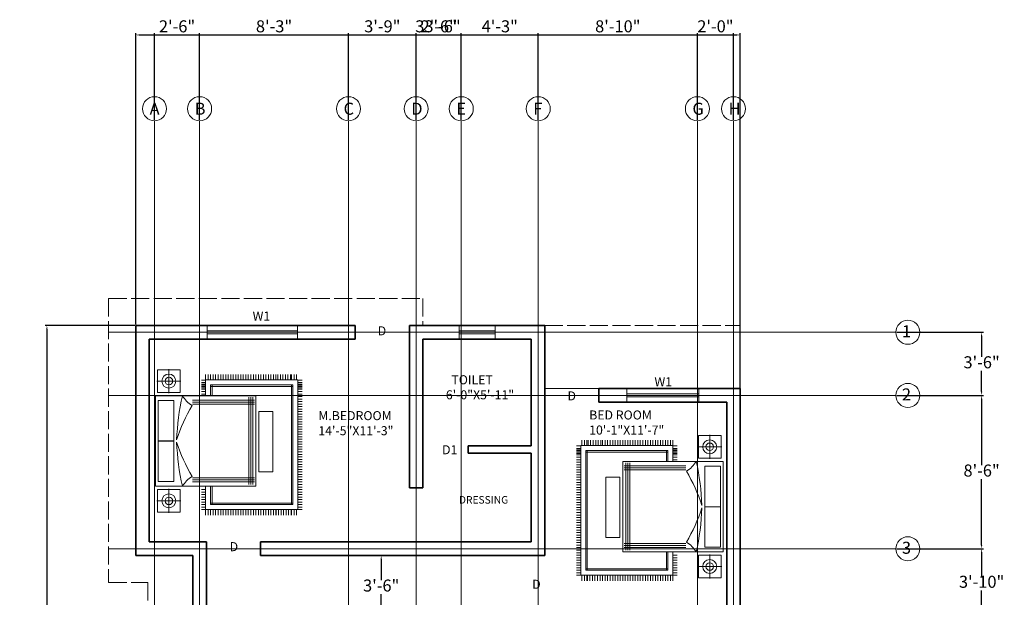
# Model space of a CAD drawing. Units: inches. Extents: x 1070 to 2371, y 645 to 1546.
# Tile 10 of 10: x 1710 to 2365, y 1162 to 1546. Entities that reach past the tile are written whole.
import ezdxf

# ---------------------------------------------------------------- set-up
doc = ezdxf.new("R2010")
doc.units = ezdxf.units.IN
doc.linetypes.add('ACAD_ISO02W100', pattern=[15, 12, -3])
for name, color, linetype, lineweight in [('A-ANNO-DIMS', 2, 'Continuous', 18), ('A-ANNO-TEXT', 7, 'Continuous', 18), ('A-AREA-IDEN', 7, 'Continuous', 18), ('A-DOOR', 4, 'Continuous', 18), ('A-FURN', 8, 'Continuous', 18), ('A-GLAZ', 4, 'Continuous', 18), ('A-GRID', 8, 'Continuous', 13), ('A-GRID-IDEN', 7, 'Continuous', 18), ('A-ROOF-OVHD', 8, 'ACAD_ISO02W100', 13), ('A-WALL', 7, 'Continuous', 35)]:
    doc.layers.add(name, color=color, linetype=linetype, lineweight=lineweight)
doc.styles.get("Standard").update_dxf_attribs({"font": 'arial.ttf'})
doc.dimstyles.new('ISO-25', dxfattribs={"dimtxt": 8, "dimasz": 2.5, "dimexe": 1.25, "dimexo": 0.625, "dimtad": 1, "dimtih": 1, "dimtoh": 1, "dimdec": 1, "dimlunit": 3, "dimtxsty": 'Standard', "dimcen": 2.5, "dimadec": 0, "dimazin": 0, "dimtfac": 1, "dimtdec": 1, "dimtmove": 0, "dimatfit": 3, "dimfxl": 1, "dimarcsym": 0})

# ---------------------------------------------------------------- blocks, each defined once
blk = doc.blocks.new('A$C462B680F')
for p, q in [((0.011, 2.874, -0.291), (0.465, 2.874, -0.291)), ((0.011, 2.424, -0.291), (0.011, 2.874, -0.291)), ((0.238, 2.649, -0.561), (0.238, 2.887, -0.561)), ((0.465, 2.874, -0.291), (0.465, 2.424, -0.291)), ((2.33, 2.918, -0.291), (0.53, 2.918, -0.291)), ((0.53, 2.918, -0.291), (0.53, 0.918, -0.291)), ((1.434, 2.861, -0.291), (0.627, 2.861, -0.291)), ((0.627, 2.861, -0.291), (0.627, 2.55, -0.291)), ((1.43, 2.861, -0.291), (1.43, 2.55, -0.291)), ((2.237, 2.861, -0.291), (1.43, 2.861, -0.291)), ((1.434, 2.55, -0.291), (1.434, 2.861, -0.291)), ((2.237, 2.55, -0.291), (2.237, 2.861, -0.291)), ((2.33, 0.918, -0.291), (2.33, 2.918, -0.291)), ((2.849, 2.874, -0.291), (2.395, 2.874, -0.291)), ((2.395, 2.874, -0.291), (2.395, 2.424, -0.291)), ((2.622, 2.649, -0.561), (2.622, 2.887, -0.561)), ((2.849, 2.424, -0.291), (2.849, 2.874, -0.291)), ((0.238, 2.649, -0.561), (0, 2.649, -0.561)), ((0.238, 2.649, -0.561), (0.238, 2.411, -0.561)), ((0.238, 2.649, -0.561), (0.476, 2.649, -0.561)), ((0.627, 2.55, -0.291), (1.434, 2.55, -0.291)), ((1.43, 2.55, -0.291), (2.237, 2.55, -0.291)), ((2.622, 2.649, -0.561), (2.384, 2.649, -0.561)), ((2.622, 2.649, -0.561), (2.622, 2.411, -0.561)), ((2.622, 2.649, -0.561), (2.861, 2.649, -0.561)), ((0.465, 2.424, -0.291), (0.011, 2.424, -0.291)), ((2.395, 2.424, -0.291), (2.849, 2.424, -0.291)), ((0.615, 2.176, -0.291), (0.615, 0.947, -0.291)), ((0.655, 2.176, -0.291), (0.655, 0.947, -0.291)), ((0.695, 2.176, -0.291), (0.695, 0.947, -0.291)), ((2.165, 2.176, -0.291), (2.165, 0.947, -0.291)), ((2.205, 2.176, -0.291), (2.205, 0.947, -0.291)), ((2.245, 2.176, -0.291), (2.245, 0.947, -0.291)), ((0.219, 1.918, -0.291), (0.219, 2, -0.291)), ((0.269, 1.918, -0.291), (0.269, 2, -0.291)), ((0.296, 1.918, -0.291), (0.296, 2, -0.291)), ((0.319, 1.918, -0.291), (0.319, 2, -0.291)), ((0.346, 1.918, -0.291), (0.346, 2, -0.291)), ((0.369, 1.918, -0.291), (0.369, 2, -0.291)), ((0.396, 1.918, -0.291), (0.396, 2, -0.291)), ((0.446, 1.918, -0.291), (0.446, 2, -0.291)), ((0.496, 1.918, -0.291), (0.496, 2, -0.291)), ((2.396, 1.918, -0.291), (2.396, 2, -0.291)), ((2.446, 1.918, -0.291), (2.446, 2, -0.291)), ((2.496, 1.918, -0.291), (2.496, 2, -0.291)), ((2.546, 1.918, -0.291), (2.546, 2, -0.291)), ((2.596, 1.918, -0.291), (2.596, 2, -0.291)), ((2.646, 1.918, -0.291), (2.646, 2, -0.291)), ((2.696, 1.918, -0.291), (2.696, 2, -0.291)), ((2.746, 1.918, -0.291), (2.746, 2, -0.291)), ((2.796, 1.918, -0.291), (2.796, 2, -0.291)), ((0.215, 1.918, -0.291), (0.105, 1.918, -0.291)), ((0.215, 1.868, -0.291), (0.105, 1.868, -0.291)), ((0.215, 1.818, -0.291), (0.105, 1.818, -0.291)), ((0.215, 1.768, -0.291), (0.105, 1.768, -0.291)), ((0.215, 1.918, -0.291), (0.215, 0.082, -0.291)), ((0.53, 1.918, -0.291), (0.215, 1.918, -0.291)), ((0.315, 1.818, -0.291), (0.315, 0.182, -0.291)), ((0.53, 1.818, -0.291), (0.315, 1.818, -0.291)), ((0.53, 1.788, -0.291), (0.315, 1.788, -0.291)), ((0.345, 1.818, -0.291), (0.345, 0.182, -0.291)), ((2.33, 1.918, -0.291), (2.796, 1.918, -0.291)), ((2.33, 1.818, -0.291), (2.696, 1.818, -0.291)), ((2.33, 1.788, -0.291), (2.696, 1.788, -0.291)), ((2.666, 1.818, -0.291), (2.666, 0.182, -0.291)), ((2.696, 1.818, -0.291), (2.696, 0.182, -0.291)), ((2.796, 1.918, -0.291), (2.796, 0.082, -0.291)), ((2.796, 1.918, -0.291), (2.906, 1.918, -0.291)), ((2.796, 1.868, -0.291), (2.906, 1.868, -0.291)), ((2.796, 1.818, -0.291), (2.906, 1.818, -0.291)), ((2.796, 1.768, -0.291), (2.906, 1.768, -0.291)), ((0.215, 1.718, -0.291), (0.105, 1.718, -0.291)), ((0.215, 1.668, -0.291), (0.105, 1.668, -0.291)), ((0.215, 1.618, -0.291), (0.105, 1.618, -0.291)), ((0.215, 1.568, -0.291), (0.105, 1.568, -0.291)), ((2.796, 1.718, -0.291), (2.906, 1.718, -0.291)), ((2.796, 1.668, -0.291), (2.906, 1.668, -0.291)), ((2.796, 1.618, -0.291), (2.906, 1.618, -0.291)), ((2.796, 1.568, -0.291), (2.906, 1.568, -0.291)), ((0.215, 1.518, -0.291), (0.105, 1.518, -0.291)), ((0.215, 1.468, -0.291), (0.105, 1.468, -0.291)), ((0.215, 1.418, -0.291), (0.105, 1.418, -0.291)), ((2.796, 1.518, -0.291), (2.906, 1.518, -0.291)), ((2.796, 1.468, -0.291), (2.906, 1.468, -0.291)), ((2.796, 1.418, -0.291), (2.906, 1.418, -0.291)), ((0.215, 1.368, -0.291), (0.105, 1.368, -0.291)), ((0.215, 1.318, -0.291), (0.105, 1.318, -0.291)), ((0.215, 1.268, -0.291), (0.105, 1.268, -0.291)), ((0.215, 1.218, -0.291), (0.105, 1.218, -0.291)), ((2.796, 1.368, -0.291), (2.906, 1.368, -0.291)), ((2.796, 1.318, -0.291), (2.906, 1.318, -0.291)), ((2.796, 1.268, -0.291), (2.906, 1.268, -0.291)), ((2.796, 1.218, -0.291), (2.906, 1.218, -0.291)), ((0.215, 1.168, -0.291), (0.105, 1.168, -0.291)), ((0.215, 1.118, -0.291), (0.105, 1.118, -0.291)), ((0.215, 1.068, -0.291), (0.105, 1.068, -0.291)), ((0.215, 1.018, -0.291), (0.105, 1.018, -0.291)), ((0.558, 1.057, -0.291), (2.299, 1.057, -0.291)), ((0.558, 1.017, -0.291), (2.299, 1.017, -0.291)), ((2.796, 1.168, -0.291), (2.906, 1.168, -0.291)), ((2.796, 1.118, -0.291), (2.906, 1.118, -0.291)), ((2.796, 1.068, -0.291), (2.906, 1.068, -0.291)), ((2.796, 1.018, -0.291), (2.906, 1.018, -0.291)), ((0.215, 0.968, -0.291), (0.105, 0.968, -0.291)), ((0.215, 0.918, -0.291), (0.105, 0.918, -0.291)), ((0.215, 0.868, -0.291), (0.105, 0.868, -0.291)), ((0.215, 0.818, -0.291), (0.105, 0.818, -0.291)), ((0.53, 0.918, -0.291), (2.33, 0.918, -0.291)), ((0.558, 0.977, -0.291), (2.299, 0.977, -0.291)), ((0.844, 0.859, -0.291), (0.844, 0.579, -0.291)), ((2.044, 0.859, -0.291), (0.844, 0.859, -0.291)), ((2.044, 0.579, -0.291), (2.044, 0.859, -0.291)), ((2.796, 0.968, -0.291), (2.906, 0.968, -0.291)), ((2.796, 0.918, -0.291), (2.906, 0.918, -0.291)), ((2.796, 0.868, -0.291), (2.906, 0.868, -0.291)), ((2.796, 0.818, -0.291), (2.906, 0.818, -0.291)), ((0.215, 0.768, -0.291), (0.105, 0.768, -0.291)), ((0.215, 0.718, -0.291), (0.105, 0.718, -0.291)), ((0.215, 0.668, -0.291), (0.105, 0.668, -0.291)), ((0.215, 0.618, -0.291), (0.105, 0.618, -0.291)), ((2.796, 0.768, -0.291), (2.906, 0.768, -0.291)), ((2.796, 0.718, -0.291), (2.906, 0.718, -0.291)), ((2.796, 0.668, -0.291), (2.906, 0.668, -0.291)), ((2.796, 0.618, -0.291), (2.906, 0.618, -0.291)), ((0.215, 0.568, -0.291), (0.105, 0.568, -0.291)), ((0.215, 0.518, -0.291), (0.105, 0.518, -0.291)), ((0.215, 0.48, -0.291), (0.105, 0.48, -0.291)), ((0.215, 0.43, -0.291), (0.105, 0.43, -0.291)), ((0.844, 0.579, -0.291), (2.044, 0.579, -0.291)), ((2.796, 0.568, -0.291), (2.906, 0.568, -0.291)), ((2.796, 0.518, -0.291), (2.906, 0.518, -0.291)), ((2.796, 0.516, -0.291), (2.906, 0.516, -0.291)), ((2.796, 0.466, -0.291), (2.906, 0.466, -0.291)), ((2.796, 0.416, -0.291), (2.906, 0.416, -0.291)), ((0.215, 0.38, -0.291), (0.105, 0.38, -0.291)), ((0.215, 0.33, -0.291), (0.105, 0.33, -0.291)), ((0.215, 0.28, -0.291), (0.105, 0.28, -0.291)), ((0.215, 0.23, -0.291), (0.105, 0.23, -0.291)), ((0.215, 0.207, -0.291), (0.105, 0.207, -0.291)), ((0.215, 0.207, -0.291), (0.105, 0.207, -0.291)), ((2.696, 0.212, -0.291), (0.315, 0.212, -0.291)), ((2.796, 0.366, -0.291), (2.906, 0.366, -0.291)), ((2.796, 0.316, -0.291), (2.906, 0.316, -0.291)), ((2.796, 0.266, -0.291), (2.906, 0.266, -0.291)), ((2.796, 0.216, -0.291), (2.906, 0.216, -0.291)), ((2.796, 0.207, -0.291), (2.906, 0.207, -0.291)), ((2.796, 0.207, -0.291), (2.906, 0.207, -0.291)), ((0.215, 0.157, -0.291), (0.105, 0.157, -0.291)), ((0.215, 0.107, -0.291), (0.105, 0.107, -0.291)), ((2.796, 0.082, -0.291), (0.215, 0.082, -0.291)), ((0.219, 0.082, -0.291), (0.219, 0, -0.291)), ((0.269, 0.082, -0.291), (0.269, 0, -0.291)), ((0.296, 0.082, -0.291), (0.296, 0, -0.291)), ((2.696, 0.182, -0.291), (0.315, 0.182, -0.291)), ((0.319, 0.082, -0.291), (0.319, 0, -0.291)), ((0.346, 0.082, -0.291), (0.346, 0, -0.291)), ((0.369, 0.082, -0.291), (0.369, 0, -0.291)), ((0.396, 0.082, -0.291), (0.396, 0, -0.291)), ((0.446, 0.082, -0.291), (0.446, 0, -0.291)), ((0.496, 0.082, -0.291), (0.496, 0, -0.291)), ((0.546, 0.082, -0.291), (0.546, 0, -0.291)), ((0.596, 0.082, -0.291), (0.596, 0, -0.291)), ((0.646, 0.082, -0.291), (0.646, 0, -0.291)), ((0.696, 0.082, -0.291), (0.696, 0, -0.291)), ((0.746, 0.082, -0.291), (0.746, 0, -0.291)), ((0.796, 0.082, -0.291), (0.796, 0, -0.291)), ((0.846, 0.082, -0.291), (0.846, 0, -0.291)), ((0.896, 0.082, -0.291), (0.896, 0, -0.291)), ((0.946, 0.082, -0.291), (0.946, 0, -0.291)), ((0.996, 0.082, -0.291), (0.996, 0, -0.291)), ((1.046, 0.082, -0.291), (1.046, 0, -0.291)), ((1.096, 0.082, -0.291), (1.096, 0, -0.291)), ((1.146, 0.082, -0.291), (1.146, 0, -0.291)), ((1.196, 0.082, -0.291), (1.196, 0, -0.291)), ((1.246, 0.082, -0.291), (1.246, 0, -0.291)), ((1.296, 0.082, -0.291), (1.296, 0, -0.291)), ((1.346, 0.082, -0.291), (1.346, 0, -0.291)), ((1.346, 0.082, -0.291), (1.346, 0, -0.291)), ((1.396, 0.082, -0.291), (1.396, 0, -0.291)), ((1.396, 0.082, -0.291), (1.396, 0, -0.291)), ((1.446, 0.082, -0.291), (1.446, 0, -0.291)), ((1.446, 0.082, -0.291), (1.446, 0, -0.291)), ((1.496, 0.082, -0.291), (1.496, 0, -0.291)), ((1.496, 0.082, -0.291), (1.496, 0, -0.291)), ((1.546, 0.082, -0.291), (1.546, 0, -0.291)), ((1.596, 0.082, -0.291), (1.596, 0, -0.291)), ((1.646, 0.082, -0.291), (1.646, 0, -0.291)), ((1.696, 0.082, -0.291), (1.696, 0, -0.291)), ((1.746, 0.082, -0.291), (1.746, 0, -0.291)), ((1.796, 0.082, -0.291), (1.796, 0, -0.291)), ((1.846, 0.082, -0.291), (1.846, 0, -0.291)), ((1.846, 0.082, -0.291), (1.846, 0, -0.291)), ((1.896, 0.082, -0.291), (1.896, 0, -0.291)), ((1.946, 0.082, -0.291), (1.946, 0, -0.291)), ((1.996, 0.082, -0.291), (1.996, 0, -0.291)), ((2.046, 0.082, -0.291), (2.046, 0, -0.291)), ((2.096, 0.082, -0.291), (2.096, 0, -0.291)), ((2.146, 0.082, -0.291), (2.146, 0, -0.291)), ((2.196, 0.082, -0.291), (2.196, 0, -0.291)), ((2.246, 0.082, -0.291), (2.246, 0, -0.291)), ((2.296, 0.082, -0.291), (2.296, 0, -0.291)), ((2.346, 0.082, -0.291), (2.346, 0, -0.291)), ((2.396, 0.082, -0.291), (2.396, 0, -0.291)), ((2.446, 0.082, -0.291), (2.446, 0, -0.291)), ((2.496, 0.082, -0.291), (2.496, 0, -0.291)), ((2.546, 0.082, -0.291), (2.546, 0, -0.291)), ((2.596, 0.082, -0.291), (2.596, 0, -0.291)), ((2.646, 0.082, -0.291), (2.646, 0, -0.291)), ((2.696, 0.082, -0.291), (2.696, 0, -0.291)), ((2.746, 0.082, -0.291), (2.746, 0, -0.291)), ((2.796, 0.157, -0.291), (2.906, 0.157, -0.291)), ((2.796, 0.107, -0.291), (2.906, 0.107, -0.291)), ((2.796, 0.082, -0.291), (2.796, 0, -0.291))]:
    blk.add_line(p, q)
for centre, radius in [((0.238, 2.649, -0.561), 0.139), ((2.622, 2.649, -0.561), 0.139), ((0.238, 2.649, -0.561), 0.075), ((2.622, 2.649, -0.561), 0.075)]:
    blk.add_circle(centre, radius)
for centre, radius, start, end in [((1.618, -2.572, -0.291), 5.071, 92.3872, 102.3913), ((0.231, 1.886, -0.291), 0.578, 31.4118, 58.8491), ((2.601, -1.074, -0.291), 3.763, 108.5127, 119.9306), ((1.243, -2.572, -0.291), 5.071, 77.6087, 87.6128), ((0.259, -1.074, -0.291), 3.763, 60.0694, 71.4873), ((2.63, 1.886, -0.291), 0.578, 121.1509, 148.5882)]:
    blk.add_arc(centre, radius, start, end)
blk = doc.blocks.new('*D16')
at = {"layer": 'A-ANNO-DIMS', "color": 0, "lineweight": -2, "transparency": 16777216}
for p, q in [((1946.48, 1189.77), (1952.04, 1189.77)), ((1950.79, 1187.27), (1950.79, 1173.48)), ((1950.79, 1150.27), (1950.79, 1164.06)), ((1946.48, 1147.77), (1952.04, 1147.77))]:
    blk.add_line(p, q, dxfattribs=at)
at = {"layer": 'A-ANNO-DIMS', "color": 0, "transparency": 16777216}
for points in [[(1950.37, 1187.27), (1951.21, 1187.27), (1950.79, 1189.77)], [(1950.37, 1150.27), (1951.21, 1150.27), (1950.79, 1147.77)]]:
    blk.add_solid(points, dxfattribs=at)
at = {"layer": 'Defpoints', "color": 0, "transparency": 16777216}
for p in [(1945.86, 1189.77), (1950.79, 1189.77), (1945.86, 1147.77)]:
    blk.add_point(p, dxfattribs=at)
at = {"layer": 'A-ANNO-DIMS', "color": 0, "transparency": 16777216, "insert": (1950.79, 1168.77), "char_height": 8, "attachment_point": 5}
blk.add_mtext('3\'-6"', dxfattribs=at)
blk = doc.blocks.new('GLAZ-48IN')
for p, q in [((0, 48), (0, 0)), ((2, 48), (2, 0))]:
    blk.add_line(p, q)
blk = doc.blocks.new('GLAZ-60IN')
for p, q in [((60, 2), (0, 2)), ((60, 0), (0, 0))]:
    blk.add_line(p, q)
blk = doc.blocks.new('GLAZ-VENT-24IN')
for p, q in [((0, 2), (24, 2)), ((0, 0), (24, 0))]:
    blk.add_line(p, q)
blk = doc.blocks.new('*D52')
at = {"layer": 'A-ANNO-DIMS', "color": 0, "lineweight": -2, "transparency": 16777216}
for p, q in [((1787.54, 1343.4), (1787.54, 1537.29)), ((1790.04, 1536.04), (2187.04, 1536.04)), ((2189.54, 1301.4), (2189.54, 1537.29))]:
    blk.add_line(p, q, dxfattribs=at)
at = {"layer": 'A-ANNO-DIMS', "color": 0, "transparency": 16777216}
for points in [[(1790.04, 1536.45), (1790.04, 1535.62), (1787.54, 1536.04)], [(2187.04, 1536.45), (2187.04, 1535.62), (2189.54, 1536.04)]]:
    blk.add_solid(points, dxfattribs=at)
at = {"layer": 'Defpoints', "color": 0, "transparency": 16777216}
for p in [(2189.54, 1536.04), (1787.54, 1342.77), (2189.54, 1300.77)]:
    blk.add_point(p, dxfattribs=at)
at = {"layer": 'A-ANNO-DIMS', "color": 0, "transparency": 16777216, "insert": (1988.54, 1540.75), "char_height": 8, "attachment_point": 5}
blk.add_mtext('33\'-6"', dxfattribs=at)
blk = doc.blocks.new('*D53')
at = {"layer": 'A-ANNO-DIMS', "color": 0, "lineweight": -2, "transparency": 16777216}
for p, q in [((1786.92, 1342.77), (1727.24, 1342.77)), ((1728.49, 1340.27), (1728.49, 1078.48)), ((1728.49, 807.27), (1728.49, 1069.06)), ((1998.92, 804.77), (1727.24, 804.77))]:
    blk.add_line(p, q, dxfattribs=at)
at = {"layer": 'A-ANNO-DIMS', "color": 0, "transparency": 16777216}
for points in [[(1728.08, 1340.27), (1728.91, 1340.27), (1728.49, 1342.77)], [(1728.08, 807.27), (1728.91, 807.27), (1728.49, 804.77)]]:
    blk.add_solid(points, dxfattribs=at)
at = {"layer": 'Defpoints', "color": 0, "transparency": 16777216}
for p in [(1787.54, 1342.77), (1728.49, 804.77), (1999.54, 804.77)]:
    blk.add_point(p, dxfattribs=at)
at = {"layer": 'A-ANNO-DIMS', "color": 0, "transparency": 16777216, "insert": (1728.49, 1073.77), "char_height": 8, "attachment_point": 5}
blk.add_mtext('44\'-10"', dxfattribs=at)
blk = doc.blocks.new('*D54')
at = {"layer": 'A-ANNO-DIMS', "color": 0, "lineweight": -2, "transparency": 16777216}
for p, q in [((1800.04, 1479.61), (1800.04, 1537.29)), ((1802.54, 1536.04), (1827.54, 1536.04)), ((1830.04, 1479.61), (1830.04, 1537.29))]:
    blk.add_line(p, q, dxfattribs=at)
at = {"layer": 'A-ANNO-DIMS', "color": 0, "transparency": 16777216}
for points in [[(1802.54, 1536.45), (1802.54, 1535.62), (1800.04, 1536.04)], [(1827.54, 1536.45), (1827.54, 1535.62), (1830.04, 1536.04)]]:
    blk.add_solid(points, dxfattribs=at)
at = {"layer": 'Defpoints', "color": 0, "transparency": 16777216}
for p in [(1830.04, 1536.04), (1800.04, 1478.99), (1830.04, 1478.99)]:
    blk.add_point(p, dxfattribs=at)
at = {"layer": 'A-ANNO-DIMS', "color": 0, "transparency": 16777216, "insert": (1815.04, 1540.74), "char_height": 8, "attachment_point": 5}
blk.add_mtext('2\'-6"', dxfattribs=at)
blk = doc.blocks.new('*D55')
at = {"layer": 'A-ANNO-DIMS', "color": 0, "lineweight": -2, "transparency": 16777216}
for p, q in [((1830.04, 1479.61), (1830.04, 1537.29)), ((1832.54, 1536.04), (1926.54, 1536.04)), ((1929.04, 1479.61), (1929.04, 1537.29))]:
    blk.add_line(p, q, dxfattribs=at)
at = {"layer": 'A-ANNO-DIMS', "color": 0, "transparency": 16777216}
for points in [[(1832.54, 1536.45), (1832.54, 1535.62), (1830.04, 1536.04)], [(1926.54, 1536.45), (1926.54, 1535.62), (1929.04, 1536.04)]]:
    blk.add_solid(points, dxfattribs=at)
at = {"layer": 'Defpoints', "color": 0, "transparency": 16777216}
for p in [(1929.04, 1536.04), (1830.04, 1478.99), (1929.04, 1478.99)]:
    blk.add_point(p, dxfattribs=at)
at = {"layer": 'A-ANNO-DIMS', "color": 0, "transparency": 16777216, "insert": (1879.54, 1540.75), "char_height": 8, "attachment_point": 5}
blk.add_mtext('8\'-3"', dxfattribs=at)
blk = doc.blocks.new('*D56')
at = {"layer": 'A-ANNO-DIMS', "color": 0, "lineweight": -2, "transparency": 16777216}
for p, q in [((1929.04, 1479.61), (1929.04, 1537.29)), ((1931.54, 1536.04), (1971.54, 1536.04)), ((1974.04, 1479.61), (1974.04, 1537.29))]:
    blk.add_line(p, q, dxfattribs=at)
at = {"layer": 'A-ANNO-DIMS', "color": 0, "transparency": 16777216}
for points in [[(1931.54, 1536.45), (1931.54, 1535.62), (1929.04, 1536.04)], [(1971.54, 1536.45), (1971.54, 1535.62), (1974.04, 1536.04)]]:
    blk.add_solid(points, dxfattribs=at)
at = {"layer": 'Defpoints', "color": 0, "transparency": 16777216}
for p in [(1974.04, 1536.04), (1929.04, 1478.99), (1974.04, 1478.99)]:
    blk.add_point(p, dxfattribs=at)
at = {"layer": 'A-ANNO-DIMS', "color": 0, "transparency": 16777216, "insert": (1951.54, 1540.75), "char_height": 8, "attachment_point": 5}
blk.add_mtext('3\'-9"', dxfattribs=at)
blk = doc.blocks.new('*D57')
at = {"layer": 'A-ANNO-DIMS', "color": 0, "lineweight": -2, "transparency": 16777216}
for p, q in [((1974.04, 1479.61), (1974.04, 1537.29)), ((1976.54, 1536.04), (2001.54, 1536.04)), ((2004.04, 1479.61), (2004.04, 1537.29))]:
    blk.add_line(p, q, dxfattribs=at)
at = {"layer": 'A-ANNO-DIMS', "color": 0, "transparency": 16777216}
for points in [[(1976.54, 1536.45), (1976.54, 1535.62), (1974.04, 1536.04)], [(2001.54, 1536.45), (2001.54, 1535.62), (2004.04, 1536.04)]]:
    blk.add_solid(points, dxfattribs=at)
at = {"layer": 'Defpoints', "color": 0, "transparency": 16777216}
for p in [(2004.04, 1536.04), (1974.04, 1478.99), (2004.04, 1478.99)]:
    blk.add_point(p, dxfattribs=at)
at = {"layer": 'A-ANNO-DIMS', "color": 0, "transparency": 16777216, "insert": (1989.04, 1540.74), "char_height": 8, "attachment_point": 5}
blk.add_mtext('2\'-6"', dxfattribs=at)
blk = doc.blocks.new('*D58')
at = {"layer": 'A-ANNO-DIMS', "color": 0, "lineweight": -2, "transparency": 16777216}
for p, q in [((2004.04, 1479.61), (2004.04, 1537.29)), ((2006.54, 1536.04), (2052.72, 1536.04)), ((2055.22, 1479.61), (2055.22, 1537.29))]:
    blk.add_line(p, q, dxfattribs=at)
at = {"layer": 'A-ANNO-DIMS', "color": 0, "transparency": 16777216}
for points in [[(2006.54, 1536.45), (2006.54, 1535.62), (2004.04, 1536.04)], [(2052.72, 1536.45), (2052.72, 1535.62), (2055.22, 1536.04)]]:
    blk.add_solid(points, dxfattribs=at)
at = {"layer": 'Defpoints', "color": 0, "transparency": 16777216}
for p in [(2055.22, 1536.04), (2004.04, 1478.99), (2055.22, 1478.99)]:
    blk.add_point(p, dxfattribs=at)
at = {"layer": 'A-ANNO-DIMS', "color": 0, "transparency": 16777216, "insert": (2029.63, 1540.75), "char_height": 8, "attachment_point": 5}
blk.add_mtext('4\'-3"', dxfattribs=at)
blk = doc.blocks.new('*D59')
at = {"layer": 'A-ANNO-DIMS', "color": 0, "lineweight": -2, "transparency": 16777216}
for p, q in [((2055.22, 1479.61), (2055.22, 1537.29)), ((2057.72, 1536.04), (2158.54, 1536.04)), ((2161.04, 1479.61), (2161.04, 1537.29))]:
    blk.add_line(p, q, dxfattribs=at)
at = {"layer": 'A-ANNO-DIMS', "color": 0, "transparency": 16777216}
for points in [[(2057.72, 1536.45), (2057.72, 1535.62), (2055.22, 1536.04)], [(2158.54, 1536.45), (2158.54, 1535.62), (2161.04, 1536.04)]]:
    blk.add_solid(points, dxfattribs=at)
at = {"layer": 'Defpoints', "color": 0, "transparency": 16777216}
for p in [(2161.04, 1536.04), (2055.22, 1478.99), (2161.04, 1478.99)]:
    blk.add_point(p, dxfattribs=at)
at = {"layer": 'A-ANNO-DIMS', "color": 0, "transparency": 16777216, "insert": (2108.13, 1540.74), "char_height": 8, "attachment_point": 5}
blk.add_mtext('8\'-10"', dxfattribs=at)
blk = doc.blocks.new('*D60')
at = {"layer": 'A-ANNO-DIMS', "color": 0, "lineweight": -2, "transparency": 16777216}
for p, q in [((2161.04, 1479.61), (2161.04, 1537.29)), ((2163.54, 1536.04), (2182.54, 1536.04)), ((2185.04, 1479.61), (2185.04, 1537.29))]:
    blk.add_line(p, q, dxfattribs=at)
at = {"layer": 'A-ANNO-DIMS', "color": 0, "transparency": 16777216}
for points in [[(2163.54, 1536.45), (2163.54, 1535.62), (2161.04, 1536.04)], [(2182.54, 1536.45), (2182.54, 1535.62), (2185.04, 1536.04)]]:
    blk.add_solid(points, dxfattribs=at)
at = {"layer": 'Defpoints', "color": 0, "transparency": 16777216}
for p in [(2185.04, 1536.04), (2161.04, 1478.99), (2185.04, 1478.99)]:
    blk.add_point(p, dxfattribs=at)
at = {"layer": 'A-ANNO-DIMS', "color": 0, "transparency": 16777216, "insert": (2173.04, 1540.74), "char_height": 8, "attachment_point": 5}
blk.add_mtext('2\'-0"', dxfattribs=at)
blk = doc.blocks.new('*D61')
at = {"layer": 'A-ANNO-DIMS', "color": 0, "lineweight": -2, "transparency": 16777216}
for p, q in [((2293.65, 1338.27), (2351.32, 1338.27)), ((2350.07, 1335.77), (2350.07, 1321.98)), ((2350.07, 1298.77), (2350.07, 1312.56)), ((2293.65, 1296.27), (2351.32, 1296.27))]:
    blk.add_line(p, q, dxfattribs=at)
at = {"layer": 'A-ANNO-DIMS', "color": 0, "transparency": 16777216}
for points in [[(2349.66, 1335.77), (2350.49, 1335.77), (2350.07, 1338.27)], [(2349.66, 1298.77), (2350.49, 1298.77), (2350.07, 1296.27)]]:
    blk.add_solid(points, dxfattribs=at)
at = {"layer": 'Defpoints', "color": 0, "transparency": 16777216}
for p in [(2293.02, 1338.27), (2293.02, 1296.27), (2350.07, 1296.27)]:
    blk.add_point(p, dxfattribs=at)
at = {"layer": 'A-ANNO-DIMS', "color": 0, "transparency": 16777216, "insert": (2350.07, 1317.27), "char_height": 8, "attachment_point": 5}
blk.add_mtext('3\'-6"', dxfattribs=at)
blk = doc.blocks.new('*D62')
at = {"layer": 'A-ANNO-DIMS', "color": 0, "lineweight": -2, "transparency": 16777216}
for p, q in [((2293.65, 1296.27), (2351.32, 1296.27)), ((2350.07, 1293.77), (2350.07, 1249.98)), ((2350.07, 1196.77), (2350.07, 1240.56)), ((2293.65, 1194.27), (2351.32, 1194.27))]:
    blk.add_line(p, q, dxfattribs=at)
at = {"layer": 'A-ANNO-DIMS', "color": 0, "transparency": 16777216}
for points in [[(2349.66, 1293.77), (2350.49, 1293.77), (2350.07, 1296.27)], [(2349.66, 1196.77), (2350.49, 1196.77), (2350.07, 1194.27)]]:
    blk.add_solid(points, dxfattribs=at)
at = {"layer": 'Defpoints', "color": 0, "transparency": 16777216}
for p in [(2293.02, 1296.27), (2293.02, 1194.27), (2350.07, 1194.27)]:
    blk.add_point(p, dxfattribs=at)
at = {"layer": 'A-ANNO-DIMS', "color": 0, "transparency": 16777216, "insert": (2350.07, 1245.27), "char_height": 8, "attachment_point": 5}
blk.add_mtext('8\'-6"', dxfattribs=at)
blk = doc.blocks.new('*D63')
at = {"layer": 'A-ANNO-DIMS', "color": 0, "lineweight": -2, "transparency": 16777216}
for p, q in [((2293.65, 1194.27), (2351.32, 1194.27)), ((2350.07, 1191.77), (2350.07, 1175.98)), ((2350.07, 1150.77), (2350.07, 1166.56)), ((2293.65, 1148.27), (2351.32, 1148.27))]:
    blk.add_line(p, q, dxfattribs=at)
at = {"layer": 'A-ANNO-DIMS', "color": 0, "transparency": 16777216}
for points in [[(2349.66, 1191.77), (2350.49, 1191.77), (2350.07, 1194.27)], [(2349.66, 1150.77), (2350.49, 1150.77), (2350.07, 1148.27)]]:
    blk.add_solid(points, dxfattribs=at)
at = {"layer": 'Defpoints', "color": 0, "transparency": 16777216}
for p in [(2293.02, 1194.27), (2293.02, 1148.27), (2350.07, 1148.27)]:
    blk.add_point(p, dxfattribs=at)
at = {"layer": 'A-ANNO-DIMS', "color": 0, "transparency": 16777216, "insert": (2350.07, 1171.27), "char_height": 8, "attachment_point": 5}
blk.add_mtext('3\'-10"', dxfattribs=at)

msp = doc.modelspace()

# ---------------------------------------------------------------- linework, layer by layer
at = {"layer": 'A-DOOR'}
msp.add_line((2095.54, 1300.77), (2059.54, 1300.77), dxfattribs=at)
at = {"layer": 'A-GLAZ'}
for p, q in [((1835.04, 1333.77), (1835.04, 1342.77)), ((1895.04, 1333.77), (1895.04, 1342.77)), ((2002.54, 1333.77), (2002.54, 1342.77)), ((2026.54, 1333.77), (2026.54, 1342.77)), ((2114.04, 1291.77), (2114.04, 1300.77)), ((2162.04, 1291.77), (2162.04, 1300.77))]:
    msp.add_line(p, q, dxfattribs=at)
at = {"layer": 'A-GRID'}
for p, q in [((1800.04, 850.77), (1800.04, 1478.99)), ((1830.04, 850.77), (1830.04, 1478.99)), ((1929.04, 850.77), (1929.04, 1478.99)), ((1974.04, 850.77), (1974.04, 1478.99)), ((2004.04, 786.77), (2004.04, 1478.99)), ((2055.22, 786.77), (2055.22, 1478.99)), ((2161.04, 786.77), (2161.04, 1478.99)), ((2185.04, 786.77), (2185.04, 1478.99)), ((1769.54, 1338.27), (2293.02, 1338.27)), ((1769.54, 1296.27), (2293.02, 1296.27)), ((1769.54, 1194.27), (2293.02, 1194.27))]:
    msp.add_line(p, q, dxfattribs=at)
at = {"layer": 'A-GRID-IDEN'}
for centre in [(1800.04, 1486.99), (1830.04, 1486.99), (1929.04, 1486.99), (1974.04, 1486.99), (2004.04, 1486.99), (2055.22, 1486.99), (2161.04, 1486.99), (2185.04, 1486.99), (2301.02, 1338.27), (2301.02, 1296.27), (2301.02, 1194.27)]:
    msp.add_circle(centre, 8, dxfattribs=at)
at = {"layer": 'A-ROOF-OVHD'}
for p, q in [((1769.54, 1360.77), (1769.54, 1171.77)), ((1769.54, 1360.77), (1978.54, 1360.77)), ((1978.54, 1360.77), (1978.54, 1342.77)), ((2059.54, 1342.77), (2189.54, 1342.77)), ((2189.54, 1342.77), (2189.54, 1300.77)), ((1769.54, 1171.77), (1795.54, 1171.77)), ((1795.54, 1171.77), (1795.54, 1007.77))]:
    msp.add_line(p, q, dxfattribs=at)
at = {"layer": 'A-WALL'}
for p, q in [((1787.54, 1342.77), (1787.54, 1189.77)), ((1787.54, 1342.77), (1933.54, 1342.77)), ((1933.54, 1342.77), (1933.54, 1333.77)), ((1969.54, 1342.77), (2059.54, 1342.77)), ((1969.54, 1342.77), (1969.54, 1234.77)), ((2059.54, 1342.77), (2059.54, 1189.77)), ((1796.54, 1333.77), (1796.54, 1198.77)), ((1796.54, 1333.77), (1933.54, 1333.77)), ((1978.54, 1333.77), (2050.54, 1333.77)), ((1978.54, 1333.77), (1978.54, 1234.77)), ((2050.54, 1333.77), (2050.54, 1262.77)), ((2095.54, 1300.77), (2189.54, 1300.77)), ((2095.54, 1300.77), (2095.54, 1291.77)), ((2189.54, 1300.77), (2189.54, 1143.77)), ((2095.54, 1291.77), (2180.54, 1291.77)), ((2180.54, 1291.77), (2180.54, 1152.77)), ((2008.54, 1262.77), (2050.54, 1262.77)), ((2008.54, 1262.77), (2008.54, 1257.77)), ((2008.54, 1257.77), (2050.54, 1257.77)), ((2050.54, 1257.77), (2050.54, 1198.77)), ((1969.54, 1234.77), (1978.54, 1234.77)), ((1796.54, 1198.77), (1834.54, 1198.77)), ((1834.54, 1198.77), (1834.54, 1043.77)), ((1870.54, 1198.77), (1969.54, 1198.77)), ((1870.54, 1198.77), (1870.54, 1189.77)), ((1969.54, 1198.77), (2050.54, 1198.77)), ((1787.54, 1189.77), (1825.54, 1189.77)), ((1825.54, 1189.77), (1825.54, 1043.77)), ((1870.54, 1189.77), (2059.54, 1189.77))]:
    msp.add_line(p, q, dxfattribs=at)

# ---------------------------------------------------------------- block references
at = {"layer": 'A-FURN', "yscale": 33.42019788357461, "zscale": 33.42019788357461}
for p, xscale, rotation in [((1898.12, 1313.75, 9.72), -33.42019788357461, 90), ((2080.72, 1270.06, 9.72), 33.42019788357461, 270)]:
    msp.add_blockref('A$C462B680F', p, dxfattribs=dict(at, xscale=xscale, rotation=rotation))
at = {"layer": 'A-GLAZ'}
for name, p in [('GLAZ-60IN', (1835.04, 1337.27)), ('GLAZ-VENT-24IN', (2002.54, 1337.27))]:
    msp.add_blockref(name, p, dxfattribs=at)
at = {"layer": 'A-GLAZ', "rotation": 90.00000000000003}
msp.add_blockref('GLAZ-48IN', (2162.05, 1295.27), dxfattribs=at)

# ---------------------------------------------------------------- texts
at = {"layer": 'A-ANNO-TEXT', "char_height": 6, "attachment_point": 1}
for s, insert in [('W1', (1865.27, 1352.09)), ('D', (1948.48, 1342.22)), ('W1', (2132.49, 1308.32)), ('D', (2074.67, 1298.96)), ('D1', (1991.28, 1263.12)), ('D', (1850, 1198.66)), ('D', (2051.21, 1173.67))]:
    msp.add_mtext_dynamic_manual_height_columns(s, width=20.5094, gutter_width=12.5, heights=[0], dxfattribs=dict(at, insert=insert))
at = {"layer": 'A-AREA-IDEN', "attachment_point": 1}
for s, width, gutter_width, heights, insert, char_height in [('  TOILET\\P6\'-0"X5\'-11"', 40.1799, 12.5, [0], (1993.8, 1309.68), 6), ('M.BEDROOM\\P14\'-5"X11\'-3"', 52.767, 12.5, [0], (1908.99, 1285.81), 6), ('BED ROOM\\P10\'-1"X11\'-7"', 101.5007, 0, [38.75], (2089.11, 1286.26), 6), ('DRESSING', 34.3208, 12.5, [0], (2002.46, 1229.31), 5)]:
    msp.add_mtext_dynamic_manual_height_columns(s, width=width, gutter_width=gutter_width, heights=heights, dxfattribs=dict(at, insert=insert, char_height=char_height))
at = {"layer": 'A-GRID-IDEN', "char_height": 8, "attachment_point": 1}
for s, insert in [('A', (1796.77, 1490.98)), ('B', (1826.77, 1490.98)), ('C', (1925.77, 1490.98)), ('D', (1970.77, 1490.98)), ('E', (2000.77, 1490.98)), ('F', (2051.95, 1490.98)), ('\\pxt4;G', (2157.77, 1490.98)), ('H', (2181.77, 1490.98)), ('1', (2297.08, 1342.93)), ('2', (2297.08, 1300.93)), ('3', (2297.08, 1198.93))]:
    msp.add_mtext_dynamic_manual_height_columns(s, width=33.3436, gutter_width=12.5, heights=[0], dxfattribs=dict(at, insert=insert))

# ---------------------------------------------------------------- dimensions: what is measured, and where the dimension line sits
at = {"layer": 'A-ANNO-DIMS'}
for base, p1, p2, picture, middle in [((2189.54, 1536.04), (1787.54, 1342.77), (2189.54, 1300.77), '*D52', (1988.54, 1540.75)), ((1830.04, 1536.04), (1800.04, 1478.99), (1830.04, 1478.99), '*D54', (1815.04, 1540.74)), ((1929.04, 1536.04), (1830.04, 1478.99), (1929.04, 1478.99), '*D55', (1879.54, 1540.75)), ((1974.04, 1536.04), (1929.04, 1478.99), (1974.04, 1478.99), '*D56', (1951.54, 1540.75)), ((2004.04, 1536.04), (1974.04, 1478.99), (2004.04, 1478.99), '*D57', (1989.04, 1540.74)), ((2055.22, 1536.04), (2004.04, 1478.99), (2055.22, 1478.99), '*D58', (2029.63, 1540.75)), ((2161.04, 1536.04), (2055.22, 1478.99), (2161.04, 1478.99), '*D59', (2108.13, 1540.74)), ((2185.04, 1536.04), (2161.04, 1478.99), (2185.04, 1478.99), '*D60', (2173.04, 1540.74))]:
    dim = msp.add_linear_dim(base=base, p1=p1, p2=p2, dimstyle='ISO-25', override={"dimdec": 1, "dimlfac": 1, "dimrnd": 0, "dimzin": 1, "dimdsep": 46, "dimlunit": 4, "dimfrac": 2}, dxfattribs=at)
    dim.commit()
    dim.dimension.update_dxf_attribs({"geometry": picture, "text_midpoint": middle})
for base, p1, p2, override, picture, middle in [((1728.49, 804.77), (1787.54, 1342.77), (1999.54, 804.77), {"dimdec": 1, "dimlfac": 1, "dimrnd": 0, "dimzin": 1, "dimdsep": 46, "dimlunit": 4, "dimfrac": 2}, '*D53', (1728.49, 1073.77)), ((2350.07, 1296.27), (2293.02, 1338.27), (2293.02, 1296.27), {"dimdec": 1, "dimlfac": 1, "dimrnd": 0, "dimzin": 1, "dimdsep": 46, "dimlunit": 4, "dimfrac": 2}, '*D61', (2350.07, 1317.27)), ((2350.07, 1194.27), (2293.02, 1296.27), (2293.02, 1194.27), {"dimdec": 1, "dimlfac": 1, "dimrnd": 0, "dimzin": 1, "dimdsep": 46, "dimlunit": 4, "dimfrac": 2}, '*D62', (2350.07, 1245.27)), ((2350.07, 1148.27), (2293.02, 1194.27), (2293.02, 1148.27), {"dimdec": 1, "dimlfac": 1, "dimrnd": 0, "dimzin": 1, "dimdsep": 46, "dimlunit": 4, "dimfrac": 2}, '*D63', (2350.07, 1171.27)), ((1950.79, 1189.77), (1945.86, 1147.77), (1945.86, 1189.77), {"dimclrd": 0, "dimclre": 0, "dimclrt": 0}, '*D16', (1950.79, 1168.77))]:
    dim = msp.add_linear_dim(base=base, p1=p1, p2=p2, angle=90, dimstyle='ISO-25', override=override, dxfattribs=at)
    dim.commit()
    dim.dimension.update_dxf_attribs({"geometry": picture, "text_midpoint": middle})

doc.saveas('drawing.dxf')
